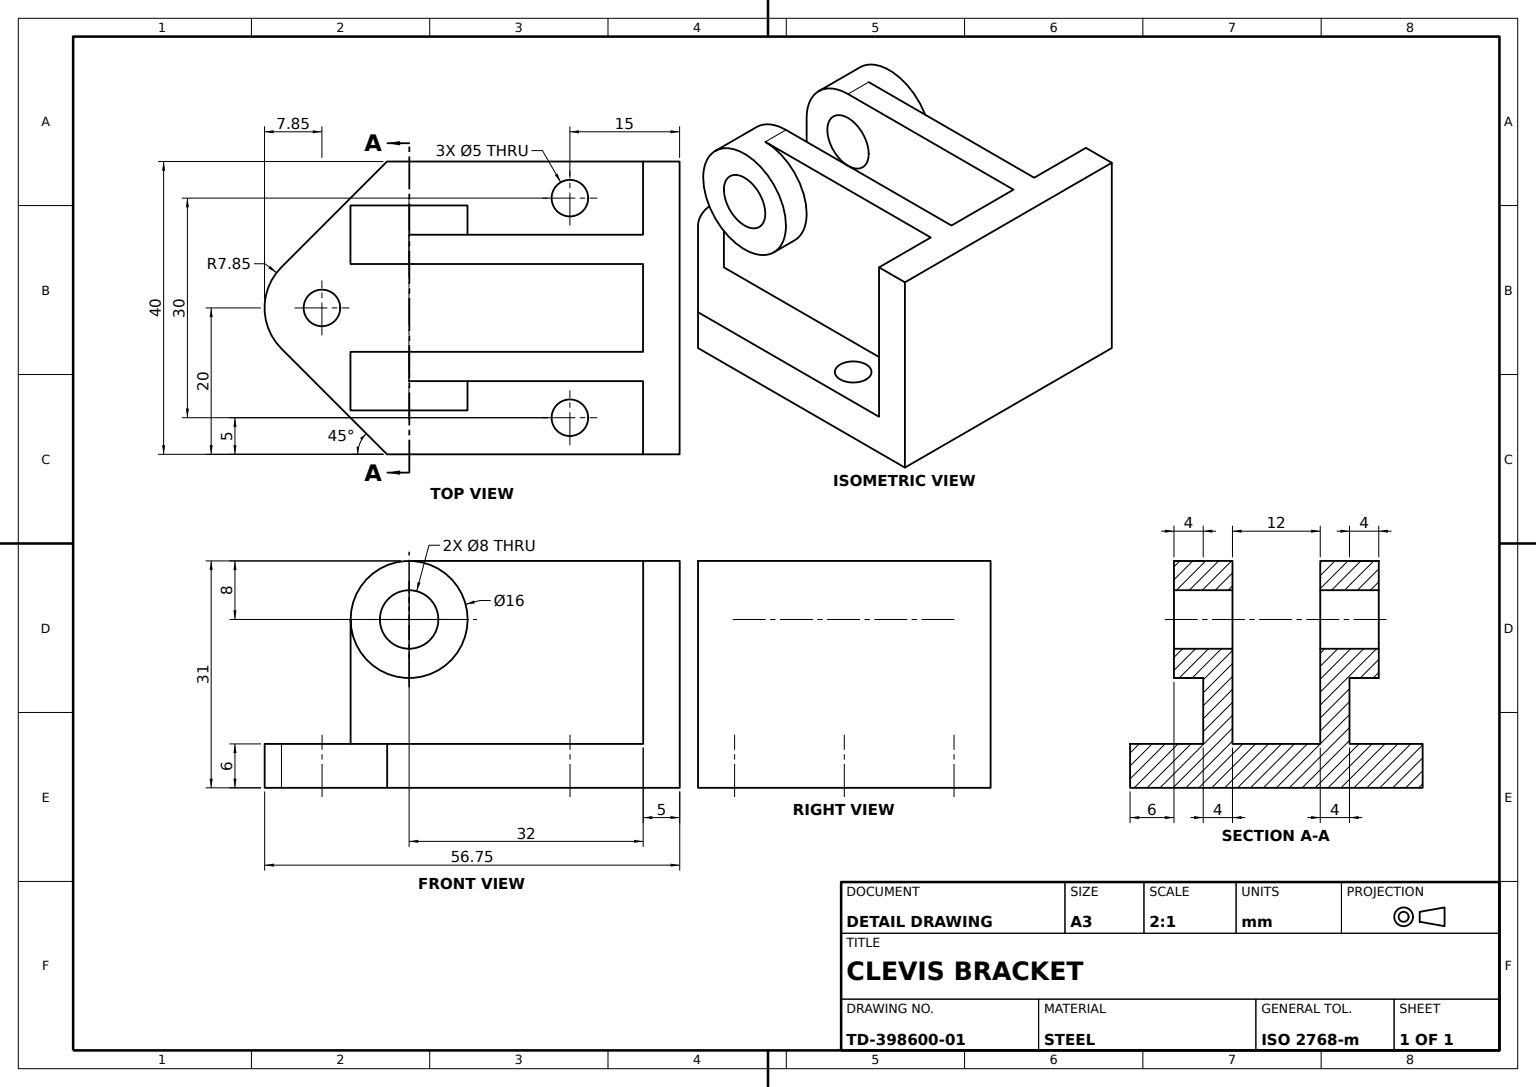
SolidWorks part; units mm, degrees
material "Plain Carbon Steel"
ref_plane "Front Plane" through (0, 0, 0) normal (0, 0, 1) x (1, 0, 0)
ref_plane "Top Plane" through (0, 0, 0) normal (0, 1, 0) x (1, 0, 0)
ref_plane "Right Plane" through (0, 0, 0) normal (1, 0, 0) x (0, 0, -1)
sketch "Base Plate Sketch" plane through (0, 0, 0) normal (0, 1, 0) x (1, 0, 0)
  line L0 (0, 0) -> (0, -48.9027) construction
  line L5 (-20, 0) -> (20, 0)
  line L6 (-20, 0) -> (-20, -40)
  line L8 (20, 0) -> (20, -40)
  line L9 (-20, -40) -> (-5.5487, -54.4513)
  line L10 (5.5487, -54.4513) -> (20, -40)
  arc A0 (-5.5487, -54.4513) -> (5.5487, -54.4513) centre (0, -48.9027) ccw
  circle A1 centre (0, -48.9027) radius 2.5
  point P11 (0, 0)
  dimension "D3" = 7.847
  dimension "D5" = 5
  dimension "D1" = 40
  dimension "D2" = 40
  dimension "D4" = 225
extrude "Pointed Base Plate" add sketch "Base Plate Sketch" along normal blind 6
sketch "Back Wall and Lugs Sketch" plane through (0, 6, 0) normal (0, 1, 0) x (1, 0, 0)
  line L0 (20, -40) -> (20, 0) construction
  line L1 (-20, 0) -> (20, 0)
  line L2 (-20, 0) -> (-20, -5)
  line L3 (-20, -5) -> (-10, -5)
  line L4 (20, 0) -> (20, -5)
  line L5 (-6, -5) -> (6, -5)
  line L7 (-10, -5) -> (-10, -45)
  line L8 (-10, -45) -> (-6, -45)
  line L9 (-6, -5) -> (-6, -45)
  line L11 (6, -5) -> (6, -45)
  line L12 (6, -45) -> (10, -45)
  line L13 (10, -5) -> (10, -45)
  line L14 (10, -5) -> (20, -5)
  line L15 (0, 0) -> (0, -5) construction
  dimension "D1" = 5
  dimension "D2" = 12
  dimension "D3" = 20
  dimension "D4" = 40
extrude "Back Wall and Clevis Lugs" add sketch "Back Wall and Lugs Sketch" along normal blind 25
sketch "Lug Boss Sketch" plane through (10, 0, 0) normal (1, 0, 0) x (0, 0, -1)
  line L0 (-45, 31) -> (-5, 31) construction
  line L1 (-45, 31) -> (-45, 6) construction
  line L2 (-5, 31) -> (-5, 6) construction
  circle A0 centre (-37, 23) radius 8
  circle A1 centre (-37, 23) radius 4
  dimension "D2" = 8
  dimension "D1" = 32
extrude "Lug Boss" add sketch "Lug Boss Sketch" along normal blind 4
sketch "Pin Hole Sketch" plane through (14, 0, 0) normal (1, 0, 0) x (0, 0, -1)
  line L0 (-45, 31) -> (-45, 23) construction
  line L1 (-45, 31) -> (-37, 31) construction
  line L2 (-45, 31) -> (-45, 23)
  line L3 (-45, 31) -> (-37, 31)
  circle A0 centre (-37, 23) radius 4 construction
  arc A1 (-37, 31) -> (-45, 23) centre (-37, 23) ccw construction
  circle A2 centre (-37, 23) radius 4
  arc A3 (-37, 31) -> (-45, 23) centre (-37, 23) ccw
extrude "Pin Hole" cut sketch "Pin Hole Sketch" against normal up to next
mirror "Lug Boss and Pin Hole Mirror" about plane through (0, 0, 0) normal (1, 0, 0) of "Pin Hole", "Lug Boss"
sketch "Mounting Holes Sketch" plane through (0, 6, 0) normal (0, 1, 0) x (1, 0, 0)
  line L0 (0, 0) -> (0, -56.7497) construction
  line L1 (20, 0) -> (-20, 0) construction
  circle A0 centre (-15, -15) radius 2.5
  arc A1 (-5.5487, -54.4513) -> (5.5487, -54.4513) centre (0, -48.9027) ccw construction
  circle A2 centre (15, -15) radius 2.5
  dimension "D3" = 5
  dimension "D1" = 30
  dimension "D2" = 15
extrude "Base Mounting Holes" cut sketch "Mounting Holes Sketch" against normal up to next
